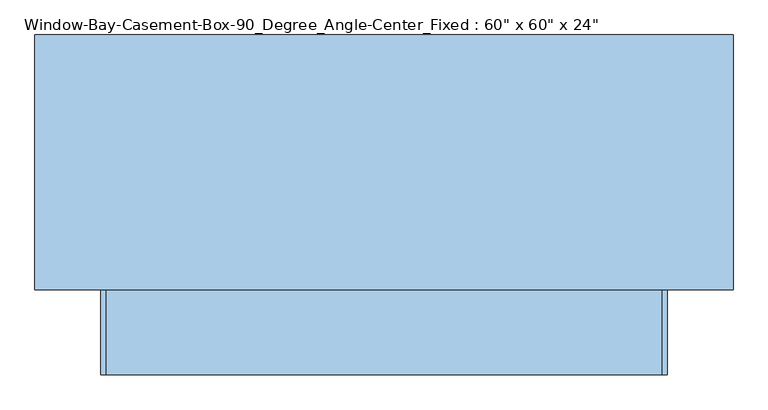
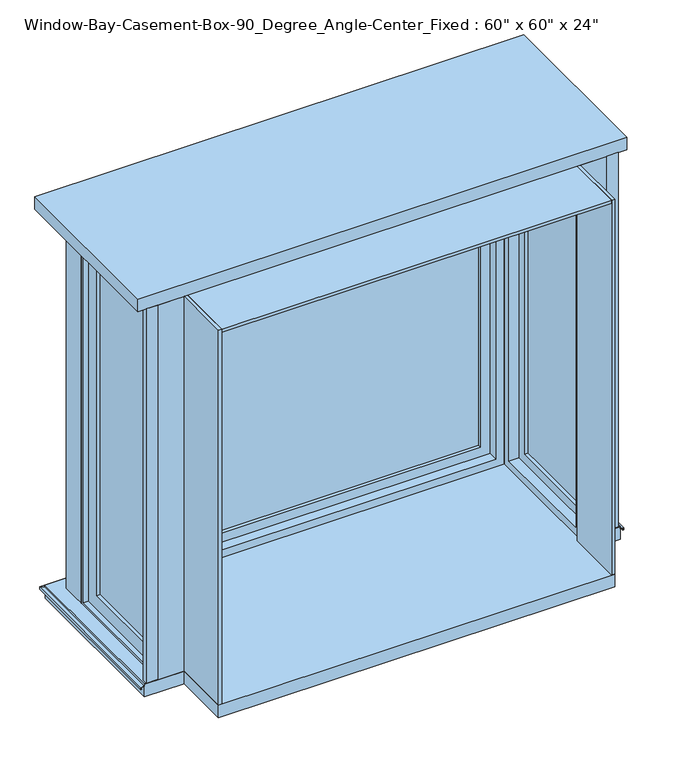
"""IFC4 building model written with IfcOpenShell, lengths in millimetres: window geometry."""

from ifc_helpers import new_model, si_unit, frame, origin, place, context, project, spatial, polyline, outline, extrude, faceted_brep, source, transform, mapped, element, save


def window_dda79932(model_context):
    return source(origin(), model_context, "Body", "SolidModel", [
        extrude(outline(polyline([(-863.6, 114.3), (-908.05, 114.3), (-908.05, 133.35), (-863.6, 133.35), (-863.6, 114.3)])), frame((0.0, 0.0, 663.1486341), z_axis=(0.0, 0.0, 1.0), x_axis=(1.0, 0.0, 0.0)), (0.0, 0.0, 1.0), 1521.2513659),
        extrude(outline(polyline([(908.05, 114.3), (863.6, 114.3), (863.6, 133.35), (908.05, 133.35), (908.05, 114.3)])), frame((0.0, 0.0, 663.1486341), z_axis=(0.0, 0.0, 1.0), x_axis=(1.0, 0.0, 0.0)), (0.0, 0.0, 1.0), 1521.2513659),
        faceted_brep([(-914.4, 114.3, 653.0697935), (-914.4, 114.3, 660.4), (-863.6, 114.3, 660.4), (-863.6, 114.3, 663.1486341), (-915.797, 114.3, 663.1486341), (-915.797, 114.3, 654.4483503), (-928.497, 114.3, 652.2089977), (-928.497, 114.3, 643.2668038), (-924.5346, 114.3, 643.2668038), (-924.5346, 114.3, 644.7270038), (-926.8968, 114.3, 644.7270038), (-926.8968, 114.3, 650.8662705), (914.4, 114.3, 653.0697935), (926.8968, 114.3, 650.8662705), (926.8968, 114.3, 644.7270038), (924.5346, 114.3, 644.7270038), (924.5346, 114.3, 643.2668038), (928.497, 114.3, 643.2668038), (928.497, 114.3, 652.2089977), (915.797, 114.3, 654.4483503), (915.797, 114.3, 663.1486341), (863.6, 114.3, 663.1486341), (863.6, 114.3, 660.4), (914.4, 114.3, 660.4), (-914.4, 774.7, 653.0697935), (-914.4, 774.7, 660.4), (914.4, 774.7, 660.4), (863.6, 723.9, 660.4), (-863.6, 723.9, 660.4), (-863.6, 723.9, 663.1486341), (863.6, 723.9, 663.1486341), (915.797, 776.097, 663.1486341), (-915.797, 776.097, 663.1486341), (-915.797, 776.097, 654.4483503), (-928.497, 788.797, 652.2089977), (-928.497, 788.797, 643.2668038), (928.497, 788.797, 643.2668038), (924.5346, 784.8346, 643.2668038), (-924.5346, 784.8346, 643.2668038), (-924.5346, 784.8346, 644.7270038), (924.5346, 784.8346, 644.7270038), (926.8968, 787.1968, 644.7270038), (-926.8968, 787.1968, 644.7270038), (-926.8968, 787.1968, 650.8662705), (914.4, 774.7, 653.0697935), (915.797, 776.097, 654.4483503), (928.497, 788.797, 652.2089977), (926.8968, 787.1968, 650.8662705)], [[[0, 1, 2, 3, 4, 5, 6, 7, 8, 9, 10, 11]], [[12, 13, 14, 15, 16, 17, 18, 19, 20, 21, 22, 23]], [[1, 0, 24, 25]], [[2, 1, 25, 26, 23, 22, 27, 28]], [[3, 2, 28, 29]], [[4, 3, 29, 30, 21, 20, 31, 32]], [[5, 4, 32, 33]], [[6, 5, 33, 34]], [[7, 6, 34, 35]], [[8, 7, 35, 36, 17, 16, 37, 38]], [[9, 8, 38, 39]], [[10, 9, 39, 40, 15, 14, 41, 42]], [[11, 10, 42, 43]], [[0, 11, 43, 24]], [[25, 24, 44, 26]], [[29, 28, 27, 30]], [[33, 32, 31, 45]], [[34, 33, 45, 46]], [[35, 34, 46, 36]], [[39, 38, 37, 40]], [[43, 42, 41, 47]], [[24, 43, 47, 44]], [[26, 44, 12, 23]], [[30, 27, 22, 21]], [[45, 31, 20, 19]], [[46, 45, 19, 18]], [[36, 46, 18, 17]], [[40, 37, 16, 15]], [[47, 41, 14, 13]], [[44, 47, 13, 12]]]),
        extrude(outline(polyline([(914.4, 774.7), (914.4, 114.3), (762.0, 114.3), (762.0, -114.3), (-762.0, -114.3), (-762.0, 114.3), (-914.4, 114.3), (-914.4, 774.7), (914.4, 774.7)])), frame((0.0, 0.0, 609.6), z_axis=(0.0, 0.0, 1.0), x_axis=(1.0, 0.0, 0.0)), (0.0, 0.0, 1.0), 50.8),
        extrude(outline(polyline([(939.8, 800.1), (939.8, 114.3), (-939.8, 114.3), (-939.8, 800.1), (939.8, 800.1)])), frame((0.0, 0.0, 2184.4), z_axis=(0.0, 0.0, 1.0), x_axis=(1.0, 0.0, 0.0)), (0.0, 0.0, 1.0), 50.8),
        extrude(outline(polyline([(-762.0, 723.9), (-762.0, 622.3), (-863.6, 622.3), (-863.6, 723.9), (-762.0, 723.9)])), frame((0.0, 0.0, 660.4), z_axis=(0.0, 0.0, 1.0), x_axis=(1.0, 0.0, 0.0)), (0.0, 0.0, 1.0), 1524.0),
        extrude(outline(polyline([(863.6, 723.9), (863.6, 622.3), (762.0, 622.3), (762.0, 723.9), (863.6, 723.9)])), frame((0.0, 0.0, 660.4), z_axis=(0.0, 0.0, 1.0), x_axis=(1.0, 0.0, 0.0)), (0.0, 0.0, 1.0), 1524.0),
        faceted_brep([(749.3, 660.4, 673.1), (749.3, 723.9, 673.1), (-749.3, 723.9, 673.1), (-749.3, 660.4, 673.1), (730.25, 622.3, 692.15), (730.25, 660.4, 692.15), (-730.25, 660.4, 692.15), (-730.25, 622.3, 692.15), (762.0, 723.9, 660.4), (762.0, 622.3, 660.4), (-762.0, 622.3, 660.4), (-762.0, 723.9, 660.4), (-749.3, 723.9, 2171.7), (-749.3, 660.4, 2171.7), (-730.25, 660.4, 2152.65), (-730.25, 622.3, 2152.65), (-762.0, 622.3, 2184.4), (-762.0, 723.9, 2184.4), (749.3, 723.9, 2171.7), (749.3, 660.4, 2171.7), (730.25, 660.4, 2152.65), (730.25, 622.3, 2152.65), (762.0, 622.3, 2184.4), (762.0, 723.9, 2184.4)], [[[0, 1, 2, 3]], [[4, 5, 6, 7]], [[8, 9, 10, 11]], [[3, 2, 12, 13]], [[7, 6, 14, 15]], [[11, 10, 16, 17]], [[13, 12, 18, 19]], [[15, 14, 20, 21]], [[17, 16, 22, 23]], [[11, 17, 23, 8], [1, 18, 12, 2]], [[19, 18, 1, 0]], [[3, 13, 19, 0], [5, 20, 14, 6]], [[21, 20, 5, 4]], [[9, 22, 16, 10], [7, 15, 21, 4]], [[23, 22, 9, 8]]]),
        extrude(outline(polyline([(2171.7, -749.3), (673.1, -749.3), (673.1, 749.3), (2171.7, 749.3), (2171.7, -749.3)]), holes=[polyline([(2114.55, 692.15), (730.25, 692.15), (730.25, -692.15), (2114.55, -692.15), (2114.55, 692.15)])]), frame((0.0, 660.4, 0.0), z_axis=(0.0, 1.0, 0.0), x_axis=(0.0, 0.0, 1.0)), (0.0, 0.0, 1.0), 44.45),
        faceted_brep([(-762.0, 146.05, 2152.65), (-800.1, 146.05, 2152.65), (-800.1, 590.55, 2152.65), (-762.0, 590.55, 2152.65), (-863.6, 114.3, 2184.4), (-762.0, 114.3, 2184.4), (-762.0, 622.3, 2184.4), (-863.6, 622.3, 2184.4), (-800.1, 127.0, 2171.7), (-863.6, 127.0, 2171.7), (-863.6, 609.6, 2171.7), (-800.1, 609.6, 2171.7), (-800.1, 590.55, 692.15), (-762.0, 590.55, 692.15), (-762.0, 622.3, 660.4), (-863.6, 622.3, 660.4), (-863.6, 609.6, 673.1), (-800.1, 609.6, 673.1), (-800.1, 146.05, 692.15), (-762.0, 146.05, 692.15), (-762.0, 114.3, 660.4), (-863.6, 114.3, 660.4), (-863.6, 127.0, 673.1), (-800.1, 127.0, 673.1)], [[[0, 1, 2, 3]], [[4, 5, 6, 7]], [[8, 9, 10, 11]], [[3, 2, 12, 13]], [[7, 6, 14, 15]], [[11, 10, 16, 17]], [[13, 12, 18, 19]], [[15, 14, 20, 21]], [[17, 16, 22, 23]], [[11, 17, 23, 8], [1, 18, 12, 2]], [[19, 18, 1, 0]], [[5, 20, 14, 6], [3, 13, 19, 0]], [[21, 20, 5, 4]], [[7, 15, 21, 4], [9, 22, 16, 10]], [[23, 22, 9, 8]]]),
        extrude(outline(polyline([(609.6, 2171.7), (609.6, 673.1), (127.0, 673.1), (127.0, 2171.7), (609.6, 2171.7)]), holes=[polyline([(184.15, 2114.55), (184.15, 730.25), (552.45, 730.25), (552.45, 2114.55), (184.15, 2114.55)])]), frame((-844.55, 0.0, 0.0), z_axis=(1.0, 0.0, 0.0), x_axis=(0.0, 1.0, 0.0)), (0.0, 0.0, 1.0), 44.45),
        faceted_brep([(800.1, 146.05, 2152.65), (762.0, 146.05, 2152.65), (762.0, 590.55, 2152.65), (800.1, 590.55, 2152.65), (863.6, 127.0, 2171.7), (800.1, 127.0, 2171.7), (800.1, 609.6, 2171.7), (863.6, 609.6, 2171.7), (762.0, 114.3, 2184.4), (863.6, 114.3, 2184.4), (863.6, 622.3, 2184.4), (762.0, 622.3, 2184.4), (762.0, 590.55, 692.15), (800.1, 590.55, 692.15), (800.1, 609.6, 673.1), (863.6, 609.6, 673.1), (863.6, 622.3, 660.4), (762.0, 622.3, 660.4), (762.0, 146.05, 692.15), (800.1, 146.05, 692.15), (800.1, 127.0, 673.1), (863.6, 127.0, 673.1), (863.6, 114.3, 660.4), (762.0, 114.3, 660.4)], [[[0, 1, 2, 3]], [[4, 5, 6, 7]], [[8, 9, 10, 11]], [[3, 2, 12, 13]], [[7, 6, 14, 15]], [[11, 10, 16, 17]], [[13, 12, 18, 19]], [[15, 14, 20, 21]], [[17, 16, 22, 23]], [[11, 17, 23, 8], [1, 18, 12, 2]], [[19, 18, 1, 0]], [[5, 20, 14, 6], [3, 13, 19, 0]], [[21, 20, 5, 4]], [[9, 22, 16, 10], [7, 15, 21, 4]], [[23, 22, 9, 8]]]),
        extrude(outline(polyline([(609.6, 2171.7), (609.6, 673.1), (127.0, 673.1), (127.0, 2171.7), (609.6, 2171.7)]), holes=[polyline([(184.15, 2114.55), (184.15, 730.25), (552.45, 730.25), (552.45, 2114.55), (184.15, 2114.55)])]), frame((800.1, 0.0, 0.0), z_axis=(1.0, 0.0, 0.0), x_axis=(0.0, 1.0, 0.0)), (0.0, 0.0, 1.0), 44.45),
        extrude(outline(polyline([(692.15, 692.15), (692.15, 685.8), (-692.15, 685.8), (-692.15, 692.15), (692.15, 692.15)])), frame((0.0, 0.0, 730.25), z_axis=(0.0, 0.0, 1.0), x_axis=(1.0, 0.0, 0.0)), (0.0, 0.0, 1.0), 1384.3),
        extrude(outline(polyline([(692.15, 679.45), (692.15, 673.1), (-692.15, 673.1), (-692.15, 679.45), (692.15, 679.45)])), frame((0.0, 0.0, 730.25), z_axis=(0.0, 0.0, 1.0), x_axis=(1.0, 0.0, 0.0)), (0.0, 0.0, 1.0), 1384.3),
        extrude(outline(polyline([(-825.5, 552.45), (-825.5, 184.15), (-831.85, 184.15), (-831.85, 552.45), (-825.5, 552.45)])), frame((0.0, 0.0, 730.25), z_axis=(0.0, 0.0, 1.0), x_axis=(1.0, 0.0, 0.0)), (0.0, 0.0, 1.0), 1384.3),
        extrude(outline(polyline([(-812.8, 552.45), (-812.8, 184.15), (-819.15, 184.15), (-819.15, 552.45), (-812.8, 552.45)])), frame((0.0, 0.0, 730.25), z_axis=(0.0, 0.0, 1.0), x_axis=(1.0, 0.0, 0.0)), (0.0, 0.0, 1.0), 1384.3),
        extrude(outline(polyline([(831.85, 552.45), (831.85, 184.15), (825.5, 184.15), (825.5, 552.45), (831.85, 552.45)])), frame((0.0, 0.0, 730.25), z_axis=(0.0, 0.0, 1.0), x_axis=(1.0, 0.0, 0.0)), (0.0, 0.0, 1.0), 1384.3),
        extrude(outline(polyline([(819.15, 552.45), (819.15, 184.15), (812.8, 184.15), (812.8, 552.45), (819.15, 552.45)])), frame((0.0, 0.0, 730.25), z_axis=(0.0, 0.0, 1.0), x_axis=(1.0, 0.0, 0.0)), (0.0, 0.0, 1.0), 1384.3),
        faceted_brep([(863.6, 127.0, 2171.7), (800.1, 127.0, 2171.7), (800.1, 609.6, 2171.7), (863.6, 609.6, 2171.7), (762.0, 114.3, 2184.4), (863.6, 114.3, 2184.4), (863.6, 622.3, 2184.4), (762.0, 622.3, 2184.4), (800.1, 146.05, 2152.65), (762.0, 146.05, 2152.65), (762.0, 590.55, 2152.65), (800.1, 590.55, 2152.65), (800.1, 609.6, 673.1), (863.6, 609.6, 673.1), (863.6, 622.3, 660.4), (762.0, 622.3, 660.4), (762.0, 590.55, 692.15), (800.1, 590.55, 692.15), (800.1, 127.0, 673.1), (863.6, 127.0, 673.1), (863.6, 114.3, 660.4), (762.0, 114.3, 660.4), (762.0, 146.05, 692.15), (800.1, 146.05, 692.15)], [[[0, 1, 2, 3]], [[4, 5, 6, 7]], [[8, 9, 10, 11]], [[3, 2, 12, 13]], [[7, 6, 14, 15]], [[11, 10, 16, 17]], [[13, 12, 18, 19]], [[15, 14, 20, 21]], [[17, 16, 22, 23]], [[1, 18, 12, 2], [11, 17, 23, 8]], [[19, 18, 1, 0]], [[5, 20, 14, 6], [3, 13, 19, 0]], [[21, 20, 5, 4]], [[7, 15, 21, 4], [9, 22, 16, 10]], [[23, 22, 9, 8]]]),
        extrude(outline(polyline([(-749.3, 114.3), (-749.3, -114.3), (-762.0, -114.3), (-762.0, 114.3), (-749.3, 114.3)])), frame((0.0, 0.0, 660.4), z_axis=(0.0, 0.0, 1.0), x_axis=(1.0, 0.0, 0.0)), (0.0, 0.0, 1.0), 1524.0),
        extrude(outline(polyline([(749.3, 114.3), (762.0, 114.3), (762.0, -114.3), (749.3, -114.3), (749.3, 114.3)])), frame((0.0, 0.0, 660.4), z_axis=(0.0, 0.0, 1.0), x_axis=(1.0, 0.0, 0.0)), (0.0, 0.0, 1.0), 1524.0),
        extrude(outline(polyline([(749.3, -114.3), (-749.3, -114.3), (-749.3, 622.3), (749.3, 622.3), (749.3, -114.3)])), frame((0.0, 0.0, 2171.7), z_axis=(0.0, 0.0, 1.0), x_axis=(1.0, 0.0, 0.0)), (0.0, 0.0, 1.0), 12.7),
    ])


if __name__ == "__main__":
    model = new_model("IFC4")
    model_context = context("Model", 3, world=origin())
    ifc_project = project(units=[si_unit("LENGTHUNIT", "METRE", prefix="MILLI")], contexts=[model_context])
    site = spatial("IfcSite", under=ifc_project)
    building = spatial("IfcBuilding", under=site)
    placement = place(None, origin())
    window_shape = window_dda79932(model_context)
    element("IfcWindow", 1, ObjectType="Window-Bay-Casement-Box-90_Degree_Angle-Center_Fixed : 60\" x 60\" x 24\"", at=placement, inside=building, context=model_context, shape_type="MappedRepresentation", body=[
        mapped(window_shape, transform((0.0, 0.0, 0.0), x_axis=(1.0, 0.0, 0.0), y_axis=(0.0, 1.0, 0.0), z_axis=(0.0, 0.0, 1.0))),
    ])
    save(model, "model.ifc")

# Revit data of these elements
# Type "Window-Bay-Casement-Box-90_Degree_Angle-Center_Fixed : 60\" x 60\" x 24\""
#   Type Mark = "18"
#   Fire Rating = "0.5h"
#   Assembly Code = "B2020100"
#   Analytic Construction = "1/8 in Pilkington single glazing"
#   Width = 5' - 0"
#   Wall Thickness [instance default] = 0' - 6"
#   Visual Light Transmittance = 0.9
#   Trim Width = 5' - 8"
#   Trim Height = 5' - 0"
#   Thermal Resistance (R) = 1.5394 (h·ft²·°F)/BTU
#   Solar Heat Gain Coefficient = 0.86
#   Rough Width = 5' - 0 1/2"
#   Rough Height = 5' - 0 1/2"
#   Height 1 = 5' - 2"
#   Height = 5' - 0"
#   Heat Transfer Coefficient (U) = 0.6496 BTU/(h·ft²·°F)
#   Depth = 2' - 0"
#   Default Sill Height = 2' - 0"
#   Side Muntin Visibility = yes
#   Center Muntin Visibility = yes
#   Interior Trim Visibility [instance default] = yes
#   Exterior Trim Visibility [instance default] = yes
#   Side Muntin Pattern = Muntin Pattern_2x2 : Muntin Pattern_2x2
#   Center Muntin Pattern = Muntin Pattern_2x2 : Muntin Pattern_2x2
#   Interior Trim Material = Wood - Stained
#   Exterior Trim Material = Clad - White
#   Exterior Trim = element 393412
#   Interior Trim = Trim-Window-Interior-Flat : Picture Frame
#   Interior Frame Material = Wood - Stained
#   Glass Panel Material = Glass
#   Exterior Frame Material = Clad - White
#   Wall Closure = (empty or 0)
# Element 1 (IfcWindow, "Window-Bay-Casement-Box-90_Degree_Angle-Center_Fixed : 60\" x 60\" x 24\"")
#   Wall Thickness = 0' - 9"
#   Materials on its faces: "Clad - White", "Wood - Stained", "Glass"
# Materials
#   "Wood - Stained": class "Wood", colour RGB 224 178 126, transparency 0, Cost = 0
#   "Clad - White": class "Wood", colour RGB 242 242 238, transparency 0, Cost = 0
#   "Glass": class "Glass", colour RGB 0 128 192, transparency 0.75, Description = "Soda Lime Glass", Cost = 0
